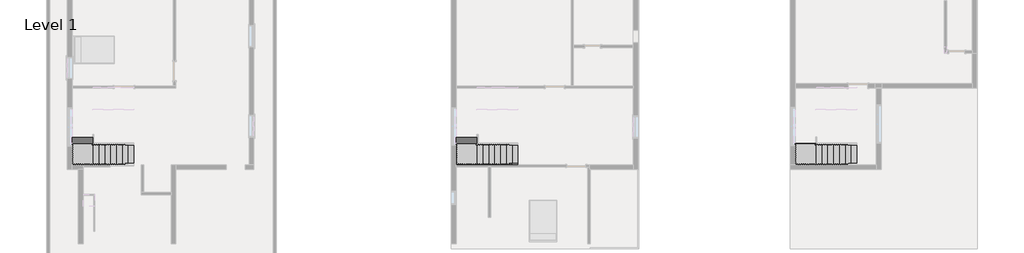
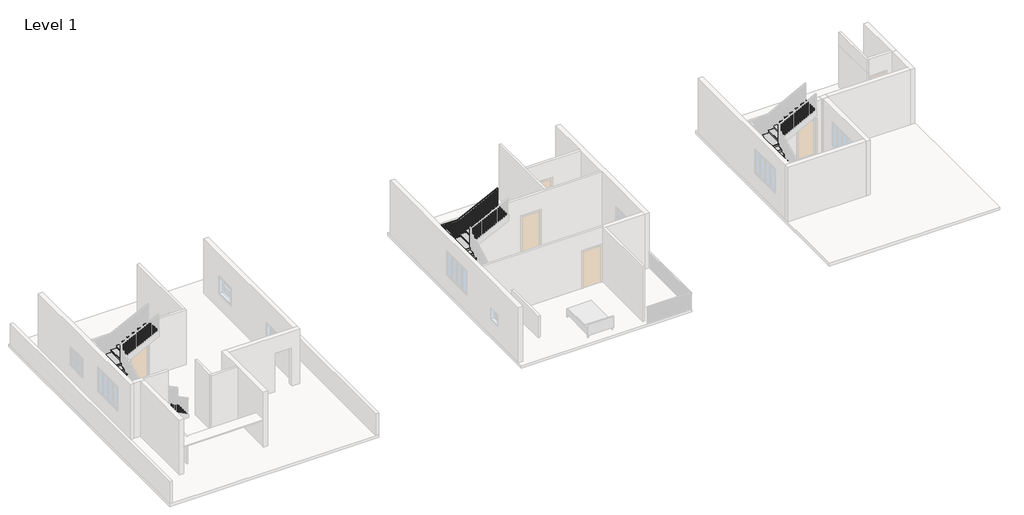
# One storey, part 5 of 8: 3 stair flights, 1 railing.
"""IFC4 building model written with IfcOpenShell, lengths in millimetres."""

from ifc_helpers import new_model, si_unit, frame, origin, place, context, project, spatial, polyline, outline, extrude, faceted_brep, transform, mapped, element, save
from components import stair_flight_046a0556, stair_flight_efd8c866, stair_flight_cb67390f

model = new_model("IFC4")

# Units and contexts
model_context = context("Model", 3, world=origin())
ifc_project = project(units=[si_unit("LENGTHUNIT", "METRE", prefix="MILLI")], contexts=[model_context])

# Site, building, storey
site = spatial("IfcSite", under=ifc_project)
building = spatial("IfcBuilding", under=site)
storey = spatial("IfcBuildingStorey", under=building, Name="Level 1", Elevation=0.0)

# Railing
placement = place(None, origin())
element("IfcRailing", 1, ObjectType="Handrail - Rectangular", at=placement, inside=storey, context=model_context, shape_type="SolidModel", body=[
    faceted_brep([(-1428.1308482, -1118.4399287, 1052.9454545), (-1428.1308482, -1118.4399287, 996.242895), (-1428.1308482, -1067.6399287, 996.242895), (-1428.1308482, -1067.6399287, 1052.9454545), (-3523.6308482, -1118.4399287, 2092.0363636), (-3535.5343434, -1118.4399287, 2041.2363636), (-3535.5343434, -1067.6399287, 2041.2363636), (-3523.6308482, -1067.6399287, 2092.0363636), (-4374.5308482, -1118.4399287, 2041.2363636), (-4374.5308482, -1118.4399287, 2092.0363636), (-4374.5308482, -267.5399287, 2092.0363636), (-4374.5308482, -255.6364336, 2041.2363636), (-4323.7308482, -1067.6399287, 2041.2363636), (-4323.7308482, -255.6364336, 2041.2363636), (-4323.7308482, -1067.6399287, 2092.0363636), (-4323.7308482, -267.5399287, 2092.0363636), (-4374.5308482, 2539.1600713, 3011.0545455), (-4374.5308482, 2539.1600713, 3061.8545455), (-3523.6308482, 2539.1600713, 3061.8545455), (-3511.7273531, 2539.1600713, 3011.0545455), (-4323.7308482, 2488.3600713, 3011.0545455), (-3511.7273531, 2488.3600713, 3011.0545455), (-4323.7308482, 2488.3600713, 3061.8545455), (-3523.6308482, 2488.3600713, 3061.8545455), (-4374.5308482, 1688.2600713, 3061.8545455), (-4374.5308482, 1700.1635664, 3011.0545455), (-4323.7308482, 1700.1635664, 3011.0545455), (-4323.7308482, 1688.2600713, 3061.8545455), (-1428.1308482, 2539.1600713, 4100.9454545), (-1428.1308482, 2488.3600713, 4100.9454545), (-1428.1308482, 2488.3600713, 4044.242895), (-1428.1308482, 2539.1600713, 4044.242895)], [[[0, 1, 2, 3]], [[1, 0, 4, 5]], [[2, 1, 5, 6]], [[3, 2, 6, 7]], [[0, 3, 7, 4]], [[8, 9, 10, 11]], [[12, 8, 11, 13]], [[14, 12, 13, 15]], [[9, 14, 15, 10]], [[16, 17, 18, 19]], [[20, 16, 19, 21]], [[22, 20, 21, 23]], [[17, 22, 23, 18]], [[5, 4, 9, 8]], [[6, 5, 8, 12]], [[7, 6, 12, 14]], [[4, 7, 14, 9]], [[11, 10, 24, 25]], [[13, 11, 25, 26]], [[15, 13, 26, 27]], [[10, 15, 27, 24]], [[25, 24, 17, 16]], [[26, 25, 16, 20]], [[27, 26, 20, 22]], [[24, 27, 22, 17]], [[28, 29, 30, 31]], [[19, 18, 28, 31]], [[21, 19, 31, 30]], [[23, 21, 30, 29]], [[18, 23, 29, 28]]]),
    extrude(outline(polyline([(4001.7346305, -1513.8558482), (3048.0, -1513.8558482), (3048.0, -1494.8058482), (4011.1809115, -1494.8058482), (4001.7346305, -1513.8558482)])), frame((0.0, 2504.2350713, 0.0), z_axis=(0.0, 1.0, 0.0), x_axis=(0.0, 0.0, 1.0)), (0.0, 0.0, 1.0), 19.05),
    extrude(outline(polyline([(3951.3544652, -1615.4558482), (3048.0, -1615.4558482), (3048.0, -1596.4058482), (3960.8007462, -1596.4058482), (3951.3544652, -1615.4558482)])), frame((0.0, 2504.2350713, 0.0), z_axis=(0.0, 1.0, 0.0), x_axis=(0.0, 0.0, 1.0)), (0.0, 0.0, 1.0), 19.05),
    extrude(outline(polyline([(3900.9742999, -1717.0558482), (3048.0, -1717.0558482), (3048.0, -1698.0058482), (3910.4205809, -1698.0058482), (3900.9742999, -1717.0558482)])), frame((0.0, 2504.2350713, 0.0), z_axis=(0.0, 1.0, 0.0), x_axis=(0.0, 0.0, 1.0)), (0.0, 0.0, 1.0), 19.05),
    extrude(outline(polyline([(3850.5941346, -1818.6558482), (2909.4545455, -1818.6558482), (2909.4545455, -1799.6058482), (3860.0404156, -1799.6058482), (3850.5941346, -1818.6558482)])), frame((0.0, 2504.2350713, 0.0), z_axis=(0.0, 1.0, 0.0), x_axis=(0.0, 0.0, 1.0)), (0.0, 0.0, 1.0), 19.05),
    extrude(outline(polyline([(3800.2139693, -1920.2558482), (2909.4545455, -1920.2558482), (2909.4545455, -1901.2058482), (3809.6602503, -1901.2058482), (3800.2139693, -1920.2558482)])), frame((0.0, 2504.2350713, 0.0), z_axis=(0.0, 1.0, 0.0), x_axis=(0.0, 0.0, 1.0)), (0.0, 0.0, 1.0), 19.05),
    extrude(outline(polyline([(3749.833804, -2021.8558482), (2770.9090909, -2021.8558482), (2770.9090909, -2002.8058482), (3759.280085, -2002.8058482), (3749.833804, -2021.8558482)])), frame((0.0, 2504.2350713, 0.0), z_axis=(0.0, 1.0, 0.0), x_axis=(0.0, 0.0, 1.0)), (0.0, 0.0, 1.0), 19.05),
    extrude(outline(polyline([(3699.4536388, -2123.4558482), (2770.9090909, -2123.4558482), (2770.9090909, -2104.4058482), (3708.8999198, -2104.4058482), (3699.4536388, -2123.4558482)])), frame((0.0, 2504.2350713, 0.0), z_axis=(0.0, 1.0, 0.0), x_axis=(0.0, 0.0, 1.0)), (0.0, 0.0, 1.0), 19.05),
    extrude(outline(polyline([(3649.0734735, -2225.0558482), (2770.9090909, -2225.0558482), (2770.9090909, -2206.0058482), (3658.5197545, -2206.0058482), (3649.0734735, -2225.0558482)])), frame((0.0, 2504.2350713, 0.0), z_axis=(0.0, 1.0, 0.0), x_axis=(0.0, 0.0, 1.0)), (0.0, 0.0, 1.0), 19.05),
    extrude(outline(polyline([(3598.6933082, -2326.6558482), (2632.3636364, -2326.6558482), (2632.3636364, -2307.6058482), (3608.1395892, -2307.6058482), (3598.6933082, -2326.6558482)])), frame((0.0, 2504.2350713, 0.0), z_axis=(0.0, 1.0, 0.0), x_axis=(0.0, 0.0, 1.0)), (0.0, 0.0, 1.0), 19.05),
    extrude(outline(polyline([(3548.3131429, -2428.2558482), (2632.3636364, -2428.2558482), (2632.3636364, -2409.2058482), (3557.7594239, -2409.2058482), (3548.3131429, -2428.2558482)])), frame((0.0, 2504.2350713, 0.0), z_axis=(0.0, 1.0, 0.0), x_axis=(0.0, 0.0, 1.0)), (0.0, 0.0, 1.0), 19.05),
    extrude(outline(polyline([(3497.9329776, -2529.8558482), (2632.3636364, -2529.8558482), (2632.3636364, -2510.8058482), (3507.3792586, -2510.8058482), (3497.9329776, -2529.8558482)])), frame((0.0, 2504.2350713, 0.0), z_axis=(0.0, 1.0, 0.0), x_axis=(0.0, 0.0, 1.0)), (0.0, 0.0, 1.0), 19.05),
    extrude(outline(polyline([(3447.5528123, -2631.4558482), (2493.8181818, -2631.4558482), (2493.8181818, -2612.4058482), (3456.9990933, -2612.4058482), (3447.5528123, -2631.4558482)])), frame((0.0, 2504.2350713, 0.0), z_axis=(0.0, 1.0, 0.0), x_axis=(0.0, 0.0, 1.0)), (0.0, 0.0, 1.0), 19.05),
    extrude(outline(polyline([(3397.172647, -2733.0558482), (2493.8181818, -2733.0558482), (2493.8181818, -2714.0058482), (3406.618928, -2714.0058482), (3397.172647, -2733.0558482)])), frame((0.0, 2504.2350713, 0.0), z_axis=(0.0, 1.0, 0.0), x_axis=(0.0, 0.0, 1.0)), (0.0, 0.0, 1.0), 19.05),
    extrude(outline(polyline([(3346.7924817, -2834.6558482), (2493.8181818, -2834.6558482), (2493.8181818, -2815.6058482), (3356.2387627, -2815.6058482), (3346.7924817, -2834.6558482)])), frame((0.0, 2504.2350713, 0.0), z_axis=(0.0, 1.0, 0.0), x_axis=(0.0, 0.0, 1.0)), (0.0, 0.0, 1.0), 19.05),
    extrude(outline(polyline([(3296.4123164, -2936.2558482), (2355.2727273, -2936.2558482), (2355.2727273, -2917.2058482), (3305.8585974, -2917.2058482), (3296.4123164, -2936.2558482)])), frame((0.0, 2504.2350713, 0.0), z_axis=(0.0, 1.0, 0.0), x_axis=(0.0, 0.0, 1.0)), (0.0, 0.0, 1.0), 19.05),
    extrude(outline(polyline([(3246.0321512, -3037.8558482), (2355.2727273, -3037.8558482), (2355.2727273, -3018.8058482), (3255.4784321, -3018.8058482), (3246.0321512, -3037.8558482)])), frame((0.0, 2504.2350713, 0.0), z_axis=(0.0, 1.0, 0.0), x_axis=(0.0, 0.0, 1.0)), (0.0, 0.0, 1.0), 19.05),
    extrude(outline(polyline([(3195.6519859, -3139.4558482), (2216.7272727, -3139.4558482), (2216.7272727, -3120.4058482), (3205.0982669, -3120.4058482), (3195.6519859, -3139.4558482)])), frame((0.0, 2504.2350713, 0.0), z_axis=(0.0, 1.0, 0.0), x_axis=(0.0, 0.0, 1.0)), (0.0, 0.0, 1.0), 19.05),
    extrude(outline(polyline([(3145.2718206, -3241.0558482), (2216.7272727, -3241.0558482), (2216.7272727, -3222.0058482), (3154.7181016, -3222.0058482), (3145.2718206, -3241.0558482)])), frame((0.0, 2504.2350713, 0.0), z_axis=(0.0, 1.0, 0.0), x_axis=(0.0, 0.0, 1.0)), (0.0, 0.0, 1.0), 19.05),
    extrude(outline(polyline([(3094.8916553, -3342.6558482), (2216.7272727, -3342.6558482), (2216.7272727, -3323.6058482), (3104.3379363, -3323.6058482), (3094.8916553, -3342.6558482)])), frame((0.0, 2504.2350713, 0.0), z_axis=(0.0, 1.0, 0.0), x_axis=(0.0, 0.0, 1.0)), (0.0, 0.0, 1.0), 19.05),
    extrude(outline(polyline([(3044.51149, -3444.2558482), (2078.1818182, -3444.2558482), (2078.1818182, -3425.2058482), (3053.957771, -3425.2058482), (3044.51149, -3444.2558482)])), frame((0.0, 2504.2350713, 0.0), z_axis=(0.0, 1.0, 0.0), x_axis=(0.0, 0.0, 1.0)), (0.0, 0.0, 1.0), 19.05),
    extrude(outline(polyline([(-3545.8558482, 2523.2850713), (-3526.8058482, 2523.2850713), (-3526.8058482, 2504.2350713), (-3545.8558482, 2504.2350713), (-3545.8558482, 2523.2850713)])), frame((0.0, 0.0, 2078.1818182), z_axis=(0.0, 0.0, 1.0), x_axis=(1.0, 0.0, 0.0)), (0.0, 0.0, 1.0), 932.8727273),
    extrude(outline(polyline([(-3647.4558482, 2523.2850713), (-3628.4058482, 2523.2850713), (-3628.4058482, 2504.2350713), (-3647.4558482, 2504.2350713), (-3647.4558482, 2523.2850713)])), frame((0.0, 0.0, 2078.1818182), z_axis=(0.0, 0.0, 1.0), x_axis=(1.0, 0.0, 0.0)), (0.0, 0.0, 1.0), 932.8727273),
    extrude(outline(polyline([(-3749.0558482, 2523.2850713), (-3730.0058482, 2523.2850713), (-3730.0058482, 2504.2350713), (-3749.0558482, 2504.2350713), (-3749.0558482, 2523.2850713)])), frame((0.0, 0.0, 2078.1818182), z_axis=(0.0, 0.0, 1.0), x_axis=(1.0, 0.0, 0.0)), (0.0, 0.0, 1.0), 932.8727273),
    extrude(outline(polyline([(-3850.6558482, 2523.2850713), (-3831.6058482, 2523.2850713), (-3831.6058482, 2504.2350713), (-3850.6558482, 2504.2350713), (-3850.6558482, 2523.2850713)])), frame((0.0, 0.0, 2078.1818182), z_axis=(0.0, 0.0, 1.0), x_axis=(1.0, 0.0, 0.0)), (0.0, 0.0, 1.0), 932.8727273),
    extrude(outline(polyline([(-3952.2558482, 2523.2850713), (-3933.2058482, 2523.2850713), (-3933.2058482, 2504.2350713), (-3952.2558482, 2504.2350713), (-3952.2558482, 2523.2850713)])), frame((0.0, 0.0, 2078.1818182), z_axis=(0.0, 0.0, 1.0), x_axis=(1.0, 0.0, 0.0)), (0.0, 0.0, 1.0), 932.8727273),
    extrude(outline(polyline([(-4053.8558482, 2523.2850713), (-4034.8058482, 2523.2850713), (-4034.8058482, 2504.2350713), (-4053.8558482, 2504.2350713), (-4053.8558482, 2523.2850713)])), frame((0.0, 0.0, 2078.1818182), z_axis=(0.0, 0.0, 1.0), x_axis=(1.0, 0.0, 0.0)), (0.0, 0.0, 1.0), 932.8727273),
    extrude(outline(polyline([(-4155.4558482, 2523.2850713), (-4136.4058482, 2523.2850713), (-4136.4058482, 2504.2350713), (-4155.4558482, 2504.2350713), (-4155.4558482, 2523.2850713)])), frame((0.0, 0.0, 2078.1818182), z_axis=(0.0, 0.0, 1.0), x_axis=(1.0, 0.0, 0.0)), (0.0, 0.0, 1.0), 932.8727273),
    extrude(outline(polyline([(-4257.0558482, 2523.2850713), (-4238.0058482, 2523.2850713), (-4238.0058482, 2504.2350713), (-4257.0558482, 2504.2350713), (-4257.0558482, 2523.2850713)])), frame((0.0, 0.0, 2078.1818182), z_axis=(0.0, 0.0, 1.0), x_axis=(1.0, 0.0, 0.0)), (0.0, 0.0, 1.0), 932.8727273),
    extrude(outline(polyline([(-4358.6558482, 2453.4350713), (-4358.6558482, 2472.4850713), (-4339.6058482, 2472.4850713), (-4339.6058482, 2453.4350713), (-4358.6558482, 2453.4350713)])), frame((0.0, 0.0, 2078.1818182), z_axis=(0.0, 0.0, 1.0), x_axis=(1.0, 0.0, 0.0)), (0.0, 0.0, 1.0), 932.8727273),
    extrude(outline(polyline([(-4358.6558482, 2351.8350713), (-4358.6558482, 2370.8850713), (-4339.6058482, 2370.8850713), (-4339.6058482, 2351.8350713), (-4358.6558482, 2351.8350713)])), frame((0.0, 0.0, 2078.1818182), z_axis=(0.0, 0.0, 1.0), x_axis=(1.0, 0.0, 0.0)), (0.0, 0.0, 1.0), 932.8727273),
    extrude(outline(polyline([(-4358.6558482, 2250.2350713), (-4358.6558482, 2269.2850713), (-4339.6058482, 2269.2850713), (-4339.6058482, 2250.2350713), (-4358.6558482, 2250.2350713)])), frame((0.0, 0.0, 2078.1818182), z_axis=(0.0, 0.0, 1.0), x_axis=(1.0, 0.0, 0.0)), (0.0, 0.0, 1.0), 932.8727273),
    extrude(outline(polyline([(-4358.6558482, 2148.6350713), (-4358.6558482, 2167.6850713), (-4339.6058482, 2167.6850713), (-4339.6058482, 2148.6350713), (-4358.6558482, 2148.6350713)])), frame((0.0, 0.0, 2078.1818182), z_axis=(0.0, 0.0, 1.0), x_axis=(1.0, 0.0, 0.0)), (0.0, 0.0, 1.0), 932.8727273),
    extrude(outline(polyline([(-4358.6558482, 2047.0350713), (-4358.6558482, 2066.0850713), (-4339.6058482, 2066.0850713), (-4339.6058482, 2047.0350713), (-4358.6558482, 2047.0350713)])), frame((0.0, 0.0, 2078.1818182), z_axis=(0.0, 0.0, 1.0), x_axis=(1.0, 0.0, 0.0)), (0.0, 0.0, 1.0), 932.8727273),
    extrude(outline(polyline([(-4358.6558482, 1945.4350713), (-4358.6558482, 1964.4850713), (-4339.6058482, 1964.4850713), (-4339.6058482, 1945.4350713), (-4358.6558482, 1945.4350713)])), frame((0.0, 0.0, 2078.1818182), z_axis=(0.0, 0.0, 1.0), x_axis=(1.0, 0.0, 0.0)), (0.0, 0.0, 1.0), 932.8727273),
    extrude(outline(polyline([(-4358.6558482, 1843.8350713), (-4358.6558482, 1862.8850713), (-4339.6058482, 1862.8850713), (-4339.6058482, 1843.8350713), (-4358.6558482, 1843.8350713)])), frame((0.0, 0.0, 2078.1818182), z_axis=(0.0, 0.0, 1.0), x_axis=(1.0, 0.0, 0.0)), (0.0, 0.0, 1.0), 932.8727273),
    extrude(outline(polyline([(-4358.6558482, 1742.2350713), (-4358.6558482, 1761.2850713), (-4339.6058482, 1761.2850713), (-4339.6058482, 1742.2350713), (-4358.6558482, 1742.2350713)])), frame((0.0, 0.0, 2078.1818182), z_axis=(0.0, 0.0, 1.0), x_axis=(1.0, 0.0, 0.0)), (0.0, 0.0, 1.0), 932.8727273),
    extrude(outline(polyline([(1659.6850713, 2990.9825644), (1659.6850713, 2078.1818182), (1640.6350713, 2078.1818182), (1640.6350713, 2981.5362834), (1659.6850713, 2990.9825644)])), frame((-4358.6558482, 0.0, 0.0), z_axis=(1.0, 0.0, 0.0), x_axis=(0.0, 1.0, 0.0)), (0.0, 0.0, 1.0), 19.05),
    extrude(outline(polyline([(1558.0850713, 2940.6023991), (1558.0850713, 2078.1818182), (1539.0350713, 2078.1818182), (1539.0350713, 2931.1561181), (1558.0850713, 2940.6023991)])), frame((-4358.6558482, 0.0, 0.0), z_axis=(1.0, 0.0, 0.0), x_axis=(0.0, 1.0, 0.0)), (0.0, 0.0, 1.0), 19.05),
    extrude(outline(polyline([(1456.4850713, 2890.2222338), (1456.4850713, 1939.6363636), (1437.4350713, 1939.6363636), (1437.4350713, 2880.7759528), (1456.4850713, 2890.2222338)])), frame((-4358.6558482, 0.0, 0.0), z_axis=(1.0, 0.0, 0.0), x_axis=(0.0, 1.0, 0.0)), (0.0, 0.0, 1.0), 19.05),
    extrude(outline(polyline([(1354.8850713, 2839.8420685), (1354.8850713, 1939.6363636), (1335.8350713, 1939.6363636), (1335.8350713, 2830.3957875), (1354.8850713, 2839.8420685)])), frame((-4358.6558482, 0.0, 0.0), z_axis=(1.0, 0.0, 0.0), x_axis=(0.0, 1.0, 0.0)), (0.0, 0.0, 1.0), 19.05),
    extrude(outline(polyline([(1253.2850713, 2789.4619032), (1253.2850713, 1801.0909091), (1234.2350713, 1801.0909091), (1234.2350713, 2780.0156222), (1253.2850713, 2789.4619032)])), frame((-4358.6558482, 0.0, 0.0), z_axis=(1.0, 0.0, 0.0), x_axis=(0.0, 1.0, 0.0)), (0.0, 0.0, 1.0), 19.05),
    extrude(outline(polyline([(1151.6850713, 2739.0817379), (1151.6850713, 1801.0909091), (1132.6350713, 1801.0909091), (1132.6350713, 2729.6354569), (1151.6850713, 2739.0817379)])), frame((-4358.6558482, 0.0, 0.0), z_axis=(1.0, 0.0, 0.0), x_axis=(0.0, 1.0, 0.0)), (0.0, 0.0, 1.0), 19.05),
    extrude(outline(polyline([(1050.0850713, 2688.7015726), (1050.0850713, 1801.0909091), (1031.0350713, 1801.0909091), (1031.0350713, 2679.2552917), (1050.0850713, 2688.7015726)])), frame((-4358.6558482, 0.0, 0.0), z_axis=(1.0, 0.0, 0.0), x_axis=(0.0, 1.0, 0.0)), (0.0, 0.0, 1.0), 19.05),
    extrude(outline(polyline([(948.4850713, 2638.3214074), (948.4850713, 1662.5454545), (929.4350713, 1662.5454545), (929.4350713, 2628.8751264), (948.4850713, 2638.3214074)])), frame((-4358.6558482, 0.0, 0.0), z_axis=(1.0, 0.0, 0.0), x_axis=(0.0, 1.0, 0.0)), (0.0, 0.0, 1.0), 19.05),
    extrude(outline(polyline([(846.8850713, 2587.9412421), (846.8850713, 1662.5454545), (827.8350713, 1662.5454545), (827.8350713, 2578.4949611), (846.8850713, 2587.9412421)])), frame((-4358.6558482, 0.0, 0.0), z_axis=(1.0, 0.0, 0.0), x_axis=(0.0, 1.0, 0.0)), (0.0, 0.0, 1.0), 19.05),
    extrude(outline(polyline([(745.2850713, 2537.5610768), (745.2850713, 1662.5454545), (726.2350713, 1662.5454545), (726.2350713, 2528.1147958), (745.2850713, 2537.5610768)])), frame((-4358.6558482, 0.0, 0.0), z_axis=(1.0, 0.0, 0.0), x_axis=(0.0, 1.0, 0.0)), (0.0, 0.0, 1.0), 19.05),
    extrude(outline(polyline([(643.6850713, 2487.1809115), (643.6850713, 1524.0), (624.6350713, 1524.0), (624.6350713, 2477.7346305), (643.6850713, 2487.1809115)])), frame((-4358.6558482, 0.0, 0.0), z_axis=(1.0, 0.0, 0.0), x_axis=(0.0, 1.0, 0.0)), (0.0, 0.0, 1.0), 19.05),
    extrude(outline(polyline([(542.0850713, 2436.8007462), (542.0850713, 1524.0), (523.0350713, 1524.0), (523.0350713, 2427.3544652), (542.0850713, 2436.8007462)])), frame((-4358.6558482, 0.0, 0.0), z_axis=(1.0, 0.0, 0.0), x_axis=(0.0, 1.0, 0.0)), (0.0, 0.0, 1.0), 19.05),
    extrude(outline(polyline([(440.4850713, 2386.4205809), (440.4850713, 1524.0), (421.4350713, 1524.0), (421.4350713, 2376.9742999), (440.4850713, 2386.4205809)])), frame((-4358.6558482, 0.0, 0.0), z_axis=(1.0, 0.0, 0.0), x_axis=(0.0, 1.0, 0.0)), (0.0, 0.0, 1.0), 19.05),
    extrude(outline(polyline([(338.8850713, 2336.0404156), (338.8850713, 1385.4545455), (319.8350713, 1385.4545455), (319.8350713, 2326.5941346), (338.8850713, 2336.0404156)])), frame((-4358.6558482, 0.0, 0.0), z_axis=(1.0, 0.0, 0.0), x_axis=(0.0, 1.0, 0.0)), (0.0, 0.0, 1.0), 19.05),
    extrude(outline(polyline([(237.2850713, 2285.6602503), (237.2850713, 1385.4545455), (218.2350713, 1385.4545455), (218.2350713, 2276.2139693), (237.2850713, 2285.6602503)])), frame((-4358.6558482, 0.0, 0.0), z_axis=(1.0, 0.0, 0.0), x_axis=(0.0, 1.0, 0.0)), (0.0, 0.0, 1.0), 19.05),
    extrude(outline(polyline([(135.6850713, 2235.280085), (135.6850713, 1246.9090909), (116.6350713, 1246.9090909), (116.6350713, 2225.833804), (135.6850713, 2235.280085)])), frame((-4358.6558482, 0.0, 0.0), z_axis=(1.0, 0.0, 0.0), x_axis=(0.0, 1.0, 0.0)), (0.0, 0.0, 1.0), 19.05),
    extrude(outline(polyline([(34.0850713, 2184.8999198), (34.0850713, 1246.9090909), (15.0350713, 1246.9090909), (15.0350713, 2175.4536388), (34.0850713, 2184.8999198)])), frame((-4358.6558482, 0.0, 0.0), z_axis=(1.0, 0.0, 0.0), x_axis=(0.0, 1.0, 0.0)), (0.0, 0.0, 1.0), 19.05),
    extrude(outline(polyline([(-67.5149287, 2134.5197545), (-67.5149287, 1246.9090909), (-86.5649287, 1246.9090909), (-86.5649287, 2125.0734735), (-67.5149287, 2134.5197545)])), frame((-4358.6558482, 0.0, 0.0), z_axis=(1.0, 0.0, 0.0), x_axis=(0.0, 1.0, 0.0)), (0.0, 0.0, 1.0), 19.05),
    extrude(outline(polyline([(-169.1149287, 2084.1395892), (-169.1149287, 1108.3636364), (-188.1649287, 1108.3636364), (-188.1649287, 2074.6933082), (-169.1149287, 2084.1395892)])), frame((-4358.6558482, 0.0, 0.0), z_axis=(1.0, 0.0, 0.0), x_axis=(0.0, 1.0, 0.0)), (0.0, 0.0, 1.0), 19.05),
    extrude(outline(polyline([(-4358.6558482, -289.7649287), (-4358.6558482, -270.7149287), (-4339.6058482, -270.7149287), (-4339.6058482, -289.7649287), (-4358.6558482, -289.7649287)])), frame((0.0, 0.0, 1108.3636364), z_axis=(0.0, 0.0, 1.0), x_axis=(1.0, 0.0, 0.0)), (0.0, 0.0, 1.0), 932.8727273),
    extrude(outline(polyline([(-4358.6558482, -391.3649287), (-4358.6558482, -372.3149287), (-4339.6058482, -372.3149287), (-4339.6058482, -391.3649287), (-4358.6558482, -391.3649287)])), frame((0.0, 0.0, 1108.3636364), z_axis=(0.0, 0.0, 1.0), x_axis=(1.0, 0.0, 0.0)), (0.0, 0.0, 1.0), 932.8727273),
    extrude(outline(polyline([(-4358.6558482, -492.9649287), (-4358.6558482, -473.9149287), (-4339.6058482, -473.9149287), (-4339.6058482, -492.9649287), (-4358.6558482, -492.9649287)])), frame((0.0, 0.0, 1108.3636364), z_axis=(0.0, 0.0, 1.0), x_axis=(1.0, 0.0, 0.0)), (0.0, 0.0, 1.0), 932.8727273),
    extrude(outline(polyline([(-4358.6558482, -594.5649287), (-4358.6558482, -575.5149287), (-4339.6058482, -575.5149287), (-4339.6058482, -594.5649287), (-4358.6558482, -594.5649287)])), frame((0.0, 0.0, 1108.3636364), z_axis=(0.0, 0.0, 1.0), x_axis=(1.0, 0.0, 0.0)), (0.0, 0.0, 1.0), 932.8727273),
    extrude(outline(polyline([(-4358.6558482, -696.1649287), (-4358.6558482, -677.1149287), (-4339.6058482, -677.1149287), (-4339.6058482, -696.1649287), (-4358.6558482, -696.1649287)])), frame((0.0, 0.0, 1108.3636364), z_axis=(0.0, 0.0, 1.0), x_axis=(1.0, 0.0, 0.0)), (0.0, 0.0, 1.0), 932.8727273),
    extrude(outline(polyline([(-4358.6558482, -797.7649287), (-4358.6558482, -778.7149287), (-4339.6058482, -778.7149287), (-4339.6058482, -797.7649287), (-4358.6558482, -797.7649287)])), frame((0.0, 0.0, 1108.3636364), z_axis=(0.0, 0.0, 1.0), x_axis=(1.0, 0.0, 0.0)), (0.0, 0.0, 1.0), 932.8727273),
    extrude(outline(polyline([(-4358.6558482, -899.3649287), (-4358.6558482, -880.3149287), (-4339.6058482, -880.3149287), (-4339.6058482, -899.3649287), (-4358.6558482, -899.3649287)])), frame((0.0, 0.0, 1108.3636364), z_axis=(0.0, 0.0, 1.0), x_axis=(1.0, 0.0, 0.0)), (0.0, 0.0, 1.0), 932.8727273),
    extrude(outline(polyline([(-4358.6558482, -1000.9649287), (-4358.6558482, -981.9149287), (-4339.6058482, -981.9149287), (-4339.6058482, -1000.9649287), (-4358.6558482, -1000.9649287)])), frame((0.0, 0.0, 1108.3636364), z_axis=(0.0, 0.0, 1.0), x_axis=(1.0, 0.0, 0.0)), (0.0, 0.0, 1.0), 932.8727273),
    extrude(outline(polyline([(-4263.4058482, -1102.5649287), (-4282.4558482, -1102.5649287), (-4282.4558482, -1083.5149287), (-4263.4058482, -1083.5149287), (-4263.4058482, -1102.5649287)])), frame((0.0, 0.0, 1108.3636364), z_axis=(0.0, 0.0, 1.0), x_axis=(1.0, 0.0, 0.0)), (0.0, 0.0, 1.0), 932.8727273),
    extrude(outline(polyline([(-4161.8058482, -1102.5649287), (-4180.8558482, -1102.5649287), (-4180.8558482, -1083.5149287), (-4161.8058482, -1083.5149287), (-4161.8058482, -1102.5649287)])), frame((0.0, 0.0, 1108.3636364), z_axis=(0.0, 0.0, 1.0), x_axis=(1.0, 0.0, 0.0)), (0.0, 0.0, 1.0), 932.8727273),
    extrude(outline(polyline([(-4060.2058482, -1102.5649287), (-4079.2558482, -1102.5649287), (-4079.2558482, -1083.5149287), (-4060.2058482, -1083.5149287), (-4060.2058482, -1102.5649287)])), frame((0.0, 0.0, 1108.3636364), z_axis=(0.0, 0.0, 1.0), x_axis=(1.0, 0.0, 0.0)), (0.0, 0.0, 1.0), 932.8727273),
    extrude(outline(polyline([(-3958.6058482, -1102.5649287), (-3977.6558482, -1102.5649287), (-3977.6558482, -1083.5149287), (-3958.6058482, -1083.5149287), (-3958.6058482, -1102.5649287)])), frame((0.0, 0.0, 1108.3636364), z_axis=(0.0, 0.0, 1.0), x_axis=(1.0, 0.0, 0.0)), (0.0, 0.0, 1.0), 932.8727273),
    extrude(outline(polyline([(-3857.0058482, -1102.5649287), (-3876.0558482, -1102.5649287), (-3876.0558482, -1083.5149287), (-3857.0058482, -1083.5149287), (-3857.0058482, -1102.5649287)])), frame((0.0, 0.0, 1108.3636364), z_axis=(0.0, 0.0, 1.0), x_axis=(1.0, 0.0, 0.0)), (0.0, 0.0, 1.0), 932.8727273),
    extrude(outline(polyline([(-3755.4058482, -1102.5649287), (-3774.4558482, -1102.5649287), (-3774.4558482, -1083.5149287), (-3755.4058482, -1083.5149287), (-3755.4058482, -1102.5649287)])), frame((0.0, 0.0, 1108.3636364), z_axis=(0.0, 0.0, 1.0), x_axis=(1.0, 0.0, 0.0)), (0.0, 0.0, 1.0), 932.8727273),
    extrude(outline(polyline([(-3653.8058482, -1102.5649287), (-3672.8558482, -1102.5649287), (-3672.8558482, -1083.5149287), (-3653.8058482, -1083.5149287), (-3653.8058482, -1102.5649287)])), frame((0.0, 0.0, 1108.3636364), z_axis=(0.0, 0.0, 1.0), x_axis=(1.0, 0.0, 0.0)), (0.0, 0.0, 1.0), 932.8727273),
    extrude(outline(polyline([(-3552.2058482, -1102.5649287), (-3571.2558482, -1102.5649287), (-3571.2558482, -1083.5149287), (-3552.2058482, -1083.5149287), (-3552.2058482, -1102.5649287)])), frame((0.0, 0.0, 1108.3636364), z_axis=(0.0, 0.0, 1.0), x_axis=(1.0, 0.0, 0.0)), (0.0, 0.0, 1.0), 932.8727273),
    extrude(outline(polyline([(2008.5693412, -3469.6558482), (1108.3636364, -3469.6558482), (1108.3636364, -3450.6058482), (1999.1230602, -3450.6058482), (2008.5693412, -3469.6558482)])), frame((0.0, -1102.5649287, 0.0), z_axis=(0.0, 1.0, 0.0), x_axis=(0.0, 0.0, 1.0)), (0.0, 0.0, 1.0), 19.05),
    extrude(outline(polyline([(1958.189176, -3368.0558482), (969.8181818, -3368.0558482), (969.8181818, -3349.0058482), (1948.742895, -3349.0058482), (1958.189176, -3368.0558482)])), frame((0.0, -1102.5649287, 0.0), z_axis=(0.0, 1.0, 0.0), x_axis=(0.0, 0.0, 1.0)), (0.0, 0.0, 1.0), 19.05),
    extrude(outline(polyline([(1907.8090107, -3266.4558482), (969.8181818, -3266.4558482), (969.8181818, -3247.4058482), (1898.3627297, -3247.4058482), (1907.8090107, -3266.4558482)])), frame((0.0, -1102.5649287, 0.0), z_axis=(0.0, 1.0, 0.0), x_axis=(0.0, 0.0, 1.0)), (0.0, 0.0, 1.0), 19.05),
    extrude(outline(polyline([(1857.4288454, -3164.8558482), (969.8181818, -3164.8558482), (969.8181818, -3145.8058482), (1847.9825644, -3145.8058482), (1857.4288454, -3164.8558482)])), frame((0.0, -1102.5649287, 0.0), z_axis=(0.0, 1.0, 0.0), x_axis=(0.0, 0.0, 1.0)), (0.0, 0.0, 1.0), 19.05),
    extrude(outline(polyline([(1807.0486801, -3063.2558482), (831.2727273, -3063.2558482), (831.2727273, -3044.2058482), (1797.6023991, -3044.2058482), (1807.0486801, -3063.2558482)])), frame((0.0, -1102.5649287, 0.0), z_axis=(0.0, 1.0, 0.0), x_axis=(0.0, 0.0, 1.0)), (0.0, 0.0, 1.0), 19.05),
    extrude(outline(polyline([(1756.6685148, -2961.6558482), (831.2727273, -2961.6558482), (831.2727273, -2942.6058482), (1747.2222338, -2942.6058482), (1756.6685148, -2961.6558482)])), frame((0.0, -1102.5649287, 0.0), z_axis=(0.0, 1.0, 0.0), x_axis=(0.0, 0.0, 1.0)), (0.0, 0.0, 1.0), 19.05),
    extrude(outline(polyline([(1706.2883495, -2860.0558482), (831.2727273, -2860.0558482), (831.2727273, -2841.0058482), (1696.8420685, -2841.0058482), (1706.2883495, -2860.0558482)])), frame((0.0, -1102.5649287, 0.0), z_axis=(0.0, 1.0, 0.0), x_axis=(0.0, 0.0, 1.0)), (0.0, 0.0, 1.0), 19.05),
    extrude(outline(polyline([(1655.9081842, -2758.4558482), (692.7272727, -2758.4558482), (692.7272727, -2739.4058482), (1646.4619032, -2739.4058482), (1655.9081842, -2758.4558482)])), frame((0.0, -1102.5649287, 0.0), z_axis=(0.0, 1.0, 0.0), x_axis=(0.0, 0.0, 1.0)), (0.0, 0.0, 1.0), 19.05),
    extrude(outline(polyline([(1605.5280189, -2656.8558482), (692.7272727, -2656.8558482), (692.7272727, -2637.8058482), (1596.0817379, -2637.8058482), (1605.5280189, -2656.8558482)])), frame((0.0, -1102.5649287, 0.0), z_axis=(0.0, 1.0, 0.0), x_axis=(0.0, 0.0, 1.0)), (0.0, 0.0, 1.0), 19.05),
    extrude(outline(polyline([(1555.1478536, -2555.2558482), (692.7272727, -2555.2558482), (692.7272727, -2536.2058482), (1545.7015726, -2536.2058482), (1555.1478536, -2555.2558482)])), frame((0.0, -1102.5649287, 0.0), z_axis=(0.0, 1.0, 0.0), x_axis=(0.0, 0.0, 1.0)), (0.0, 0.0, 1.0), 19.05),
    extrude(outline(polyline([(1504.7676883, -2453.6558482), (554.1818182, -2453.6558482), (554.1818182, -2434.6058482), (1495.3214074, -2434.6058482), (1504.7676883, -2453.6558482)])), frame((0.0, -1102.5649287, 0.0), z_axis=(0.0, 1.0, 0.0), x_axis=(0.0, 0.0, 1.0)), (0.0, 0.0, 1.0), 19.05),
    extrude(outline(polyline([(1454.3875231, -2352.0558482), (554.1818182, -2352.0558482), (554.1818182, -2333.0058482), (1444.9412421, -2333.0058482), (1454.3875231, -2352.0558482)])), frame((0.0, -1102.5649287, 0.0), z_axis=(0.0, 1.0, 0.0), x_axis=(0.0, 0.0, 1.0)), (0.0, 0.0, 1.0), 19.05),
    extrude(outline(polyline([(1404.0073578, -2250.4558482), (415.6363636, -2250.4558482), (415.6363636, -2231.4058482), (1394.5610768, -2231.4058482), (1404.0073578, -2250.4558482)])), frame((0.0, -1102.5649287, 0.0), z_axis=(0.0, 1.0, 0.0), x_axis=(0.0, 0.0, 1.0)), (0.0, 0.0, 1.0), 19.05),
    extrude(outline(polyline([(1353.6271925, -2148.8558482), (415.6363636, -2148.8558482), (415.6363636, -2129.8058482), (1344.1809115, -2129.8058482), (1353.6271925, -2148.8558482)])), frame((0.0, -1102.5649287, 0.0), z_axis=(0.0, 1.0, 0.0), x_axis=(0.0, 0.0, 1.0)), (0.0, 0.0, 1.0), 19.05),
    extrude(outline(polyline([(1303.2470272, -2047.2558482), (415.6363636, -2047.2558482), (415.6363636, -2028.2058482), (1293.8007462, -2028.2058482), (1303.2470272, -2047.2558482)])), frame((0.0, -1102.5649287, 0.0), z_axis=(0.0, 1.0, 0.0), x_axis=(0.0, 0.0, 1.0)), (0.0, 0.0, 1.0), 19.05),
    extrude(outline(polyline([(1252.8668619, -1945.6558482), (277.0909091, -1945.6558482), (277.0909091, -1926.6058482), (1243.4205809, -1926.6058482), (1252.8668619, -1945.6558482)])), frame((0.0, -1102.5649287, 0.0), z_axis=(0.0, 1.0, 0.0), x_axis=(0.0, 0.0, 1.0)), (0.0, 0.0, 1.0), 19.05),
    extrude(outline(polyline([(1202.4866966, -1844.0558482), (277.0909091, -1844.0558482), (277.0909091, -1825.0058482), (1193.0404156, -1825.0058482), (1202.4866966, -1844.0558482)])), frame((0.0, -1102.5649287, 0.0), z_axis=(0.0, 1.0, 0.0), x_axis=(0.0, 0.0, 1.0)), (0.0, 0.0, 1.0), 19.05),
    extrude(outline(polyline([(1152.1065313, -1742.4558482), (277.0909091, -1742.4558482), (277.0909091, -1723.4058482), (1142.6602503, -1723.4058482), (1152.1065313, -1742.4558482)])), frame((0.0, -1102.5649287, 0.0), z_axis=(0.0, 1.0, 0.0), x_axis=(0.0, 0.0, 1.0)), (0.0, 0.0, 1.0), 19.05),
    extrude(outline(polyline([(1101.726366, -1640.8558482), (138.5454545, -1640.8558482), (138.5454545, -1621.8058482), (1092.280085, -1621.8058482), (1101.726366, -1640.8558482)])), frame((0.0, -1102.5649287, 0.0), z_axis=(0.0, 1.0, 0.0), x_axis=(0.0, 0.0, 1.0)), (0.0, 0.0, 1.0), 19.05),
    extrude(outline(polyline([(1051.3462007, -1539.2558482), (138.5454545, -1539.2558482), (138.5454545, -1520.2058482), (1041.8999198, -1520.2058482), (1051.3462007, -1539.2558482)])), frame((0.0, -1102.5649287, 0.0), z_axis=(0.0, 1.0, 0.0), x_axis=(0.0, 0.0, 1.0)), (0.0, 0.0, 1.0), 19.05),
    extrude(outline(polyline([(-4358.6558482, 2504.2350713), (-4358.6558482, 2523.2850713), (-4339.6058482, 2523.2850713), (-4339.6058482, 2504.2350713), (-4358.6558482, 2504.2350713)])), frame((0.0, 0.0, 2078.1818182), z_axis=(0.0, 0.0, 1.0), x_axis=(1.0, 0.0, 0.0)), (0.0, 0.0, 1.0), 932.8727273),
    extrude(outline(polyline([(-4339.6058482, -1102.5649287), (-4358.6558482, -1102.5649287), (-4358.6558482, -1083.5149287), (-4339.6058482, -1083.5149287), (-4339.6058482, -1102.5649287)])), frame((0.0, 0.0, 1108.3636364), z_axis=(0.0, 0.0, 1.0), x_axis=(1.0, 0.0, 0.0)), (0.0, 0.0, 1.0), 932.8727273),
    extrude(outline(polyline([(4034.796614, -1447.1808482), (3048.0, -1447.1808482), (3048.0, -1428.1308482), (4044.242895, -1428.1308482), (4034.796614, -1447.1808482)])), frame((0.0, 2504.2350713, 0.0), z_axis=(0.0, 1.0, 0.0), x_axis=(0.0, 0.0, 1.0)), (0.0, 0.0, 1.0), 19.05),
    extrude(outline(polyline([(1005.689176, -1447.1808482), (138.5454545, -1447.1808482), (138.5454545, -1428.1308482), (996.242895, -1428.1308482), (1005.689176, -1447.1808482)])), frame((0.0, -1102.5649287, 0.0), z_axis=(0.0, 1.0, 0.0), x_axis=(0.0, 0.0, 1.0)), (0.0, 0.0, 1.0), 19.05),
])

# Stair flights
stair_flight_shape = stair_flight_046a0556(model_context)
element("IfcStairFlight", 2, ObjectType="2\" Tread 1\" Nosing 1/4\" Riser", at=placement, inside=storey, context=model_context, shape_type="MappedRepresentation", body=[
    mapped(stair_flight_shape, transform((0.0, 0.0, 0.0), x_axis=(1.0, 0.0, 0.0), y_axis=(0.0, 1.0, 0.0), z_axis=(0.0, 0.0, 1.0))),
])
stair_flight_2_shape = stair_flight_efd8c866(model_context)
element("IfcStairFlight", 3, ObjectType="2\" Tread 1\" Nosing 1/4\" Riser", at=placement, inside=storey, context=model_context, shape_type="MappedRepresentation", body=[
    mapped(stair_flight_2_shape, transform((0.0, 0.0, 0.0), x_axis=(1.0, 0.0, 0.0), y_axis=(0.0, 1.0, 0.0), z_axis=(0.0, 0.0, 1.0))),
])
stair_flight_3_shape = stair_flight_cb67390f(model_context)
element("IfcStairFlight", 4, ObjectType="2\" Tread 1\" Nosing 1/4\" Riser", at=placement, inside=storey, context=model_context, shape_type="MappedRepresentation", body=[
    mapped(stair_flight_3_shape, transform((0.0, 0.0, 0.0), x_axis=(1.0, 0.0, 0.0), y_axis=(0.0, 1.0, 0.0), z_axis=(0.0, 0.0, 1.0))),
])

save(model, "model.ifc")

# Revit data of these elements
# Type "Handrail - Rectangular"
#   Assembly Code = "C2010400"
#   built-in parameter 1008612 = 0.0416667 (stored number, unit not read)
#   built-in parameter 1008611 = 0.0416667 (stored number, unit not read)
#   built-in parameter 1008609 = 0.333333 (stored number, unit not read)
#   built-in parameter 1008604 = 0.166667 (stored number, unit not read)
#   built-in parameter 1008603 = 0.166667 (stored number, unit not read)
#   Railing Height = 3' - 0"
#   built-in parameter 1008630 = 2
#   built-in parameter 1008610 = 2
#   built-in parameter 1008618 = Baluster - Square : 3/4"
# Element 1 (IfcRailing, "Handrail - Rectangular")
#   Phase Created = New Construction
# Elements 2, 3, 4 (IfcStairFlight, "2\" Tread 1\" Nosing 1/4\" Riser")
#   Phase Created = New Construction
